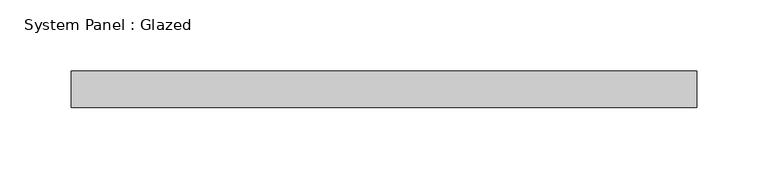
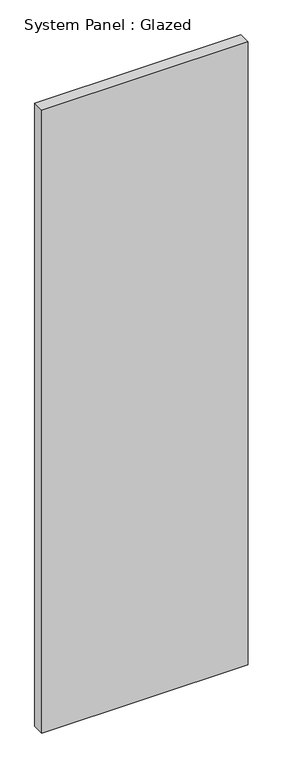
"""IFC4 building model written with IfcOpenShell, lengths in millimetres: plate geometry, System Panel : Glazed."""

from ifc_helpers import new_model, si_unit, origin, origin_with_axes, place, context, project, spatial, polyline, outline, extrude, source, transform, mapped, element, save


def system_panel_glazed_04bc9dae(model_context):
    return source(origin(), model_context, "Body", "SweptSolid", [
        extrude(outline(polyline([(219.075, 19.05), (-219.075, 19.05), (-219.075, 44.45), (219.075, 44.45), (219.075, 19.05)])), origin_with_axes(), (0.0, 0.0, 1.0), 1397.0),
    ])


if __name__ == "__main__":
    model = new_model("IFC4")
    model_context = context("Model", 3, world=origin())
    ifc_project = project(units=[si_unit("LENGTHUNIT", "METRE", prefix="MILLI")], contexts=[model_context])
    site = spatial("IfcSite", under=ifc_project)
    building = spatial("IfcBuilding", under=site)
    placement = place(None, origin())
    system_panel_glazed_shape = system_panel_glazed_04bc9dae(model_context)
    element("IfcPlate", 1, ObjectType="System Panel : Glazed", at=placement, inside=building, context=model_context, shape_type="MappedRepresentation", body=[
        mapped(system_panel_glazed_shape, transform((0.0, 0.0, 0.0), x_axis=(1.0, 0.0, 0.0), y_axis=(0.0, 1.0, 0.0), z_axis=(0.0, 0.0, 1.0))),
    ])
    save(model, "model.ifc")

# Revit data of these elements
# Type "System Panel : Glazed"
#   Construction Type Id = "GSP4R"
#   Analytic Construction = "1/8 in Pilkington single glazing"
#   Visual Light Transmittance = 0.9
#   Solar Heat Gain Coefficient = 0.86
#   Heat Transfer Coefficient (U) = 1.18115 BTU/(h·ft²·°F)
#   Define Thermal Properties by = 1
# Element 1 (IfcPlate, "System Panel : Glazed")
#   Materials on its faces: "Glass"
# Materials
#   "Glass": class "Glass", colour RGB 0 128 192, transparency 0.75, Description = "Soda Lime Glass", Cost = 0
